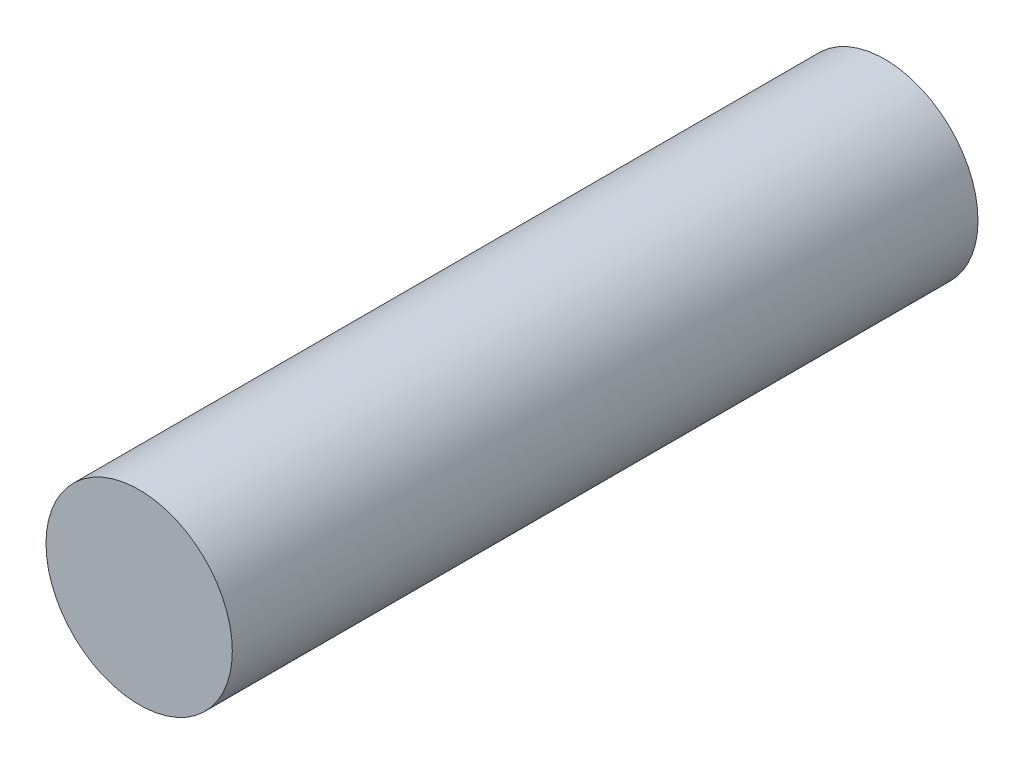
from build123d import *

# Parameters (mm, degrees)
PIN_PROFILE_9_52_R   = 4.76
PIN_BODY_L38_1_DEPTH = 38.1


with BuildPart() as part:
    # Pin Profile Ø9.52 → Pin Body L38.1 (new body)
    with BuildSketch(Plane.XY):
        with Locations(Location((0, 0, 0), (0, 0, 180))):
            Circle(PIN_PROFILE_9_52_R)
    extrude(amount=PIN_BODY_L38_1_DEPTH)


solid = part.part
